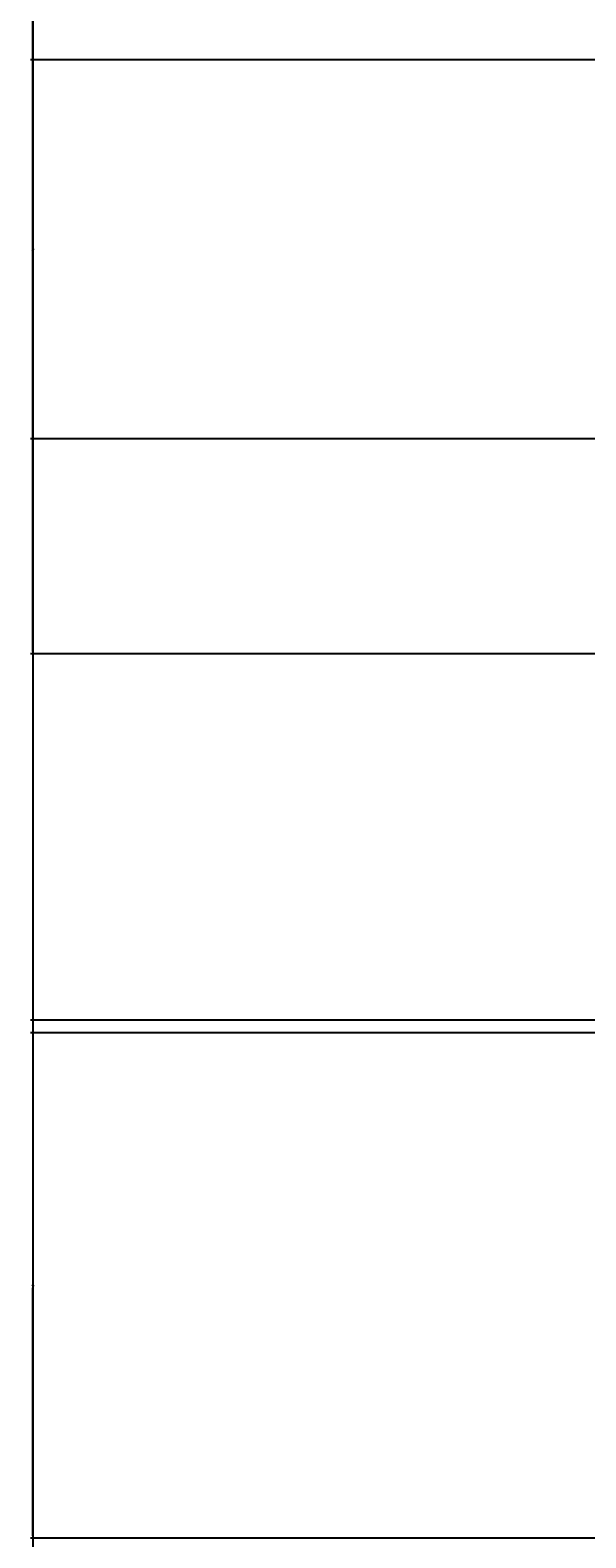
# Model space of a CAD drawing. Units: feet. Extents: x 105 to 1094, y -88 to 588.
# Tile 21 of 59: x 105 to 149, y 354 to 473. Entities that reach past the tile are written whole.
import ezdxf

# ---------------------------------------------------------------- set-up
doc = ezdxf.new("R2010")
doc.units = ezdxf.units.FT
doc.header["$MEASUREMENT"] = 0
doc.layers.add('A-ANNO-DIMS', color=2, linetype='Continuous', lineweight=18)
doc.styles.get("Standard").update_dxf_attribs({"font": 'arial.ttf'})
doc.dimstyles.get("Standard").update_dxf_attribs({"dimtxt": 0.18, "dimasz": 0.18, "dimexe": 0.18, "dimexo": 0.0625, "dimgap": 0.09, "dimtad": 0, "dimtih": 1, "dimtoh": 1, "dimdec": 4, "dimzin": 0, "dimdsep": 46, "dimtxsty": 'Standard', "dimcen": 0.09, "dimadec": 0, "dimazin": 0, "dimtfac": 1, "dimtdec": 4, "dimtofl": 0, "dimtmove": 0, "dimatfit": 3, "dimfxl": 1, "dimtolj": 1, "dimtzin": 0, "dimarcsym": 0})

# ---------------------------------------------------------------- blocks, each defined once
blk = doc.blocks.new('*D21')
at = {"layer": 'A-ANNO-DIMS', "color": 0, "lineweight": -2, "transparency": 16777216}
for p, q in [((849.63, 543.08), (105.46, 543.08)), ((105.64, 542.9), (105.64, 250.26)), ((105.64, -42.74), (105.64, 249.9)), ((849.63, -42.92), (105.46, -42.92))]:
    blk.add_line(p, q, dxfattribs=at)
at = {"layer": 'A-ANNO-DIMS', "color": 0, "transparency": 16777216}
for points in [[(105.61, 542.9), (105.67, 542.9), (105.64, 543.08)], [(105.61, -42.74), (105.67, -42.74), (105.64, -42.92)]]:
    blk.add_solid(points, dxfattribs=at)
at = {"layer": 'Defpoints', "color": 0, "transparency": 16777216}
for p in [(105.64, 543.08), (849.69, 543.08), (849.69, -42.92)]:
    blk.add_point(p, dxfattribs=at)
at = {"layer": 'A-ANNO-DIMS', "color": 0, "transparency": 16777216, "insert": (105.64, 250.08), "char_height": 0.18, "attachment_point": 5}
blk.add_mtext('\\A1;586', dxfattribs=at)
blk = doc.blocks.new('*D27')
at = {"layer": 'A-ANNO-DIMS', "color": 0, "lineweight": -2, "transparency": 16777216}
for p, q in [((231.63, 543.08), (105.46, 543.08)), ((105.64, 542.9), (105.64, 483.76)), ((105.64, 424.26), (105.64, 483.4)), ((150.63, 424.08), (105.46, 424.08))]:
    blk.add_line(p, q, dxfattribs=at)
at = {"layer": 'A-ANNO-DIMS', "color": 0, "transparency": 16777216}
for points in [[(105.61, 542.9), (105.67, 542.9), (105.64, 543.08)], [(105.61, 424.26), (105.67, 424.26), (105.64, 424.08)]]:
    blk.add_solid(points, dxfattribs=at)
at = {"layer": 'Defpoints', "color": 0, "transparency": 16777216}
for p in [(105.64, 543.08), (231.69, 543.08), (150.69, 424.08)]:
    blk.add_point(p, dxfattribs=at)
at = {"layer": 'A-ANNO-DIMS', "color": 0, "transparency": 16777216, "insert": (105.64, 483.58), "char_height": 0.18, "attachment_point": 5}
blk.add_mtext('\\A1;119', dxfattribs=at)
blk = doc.blocks.new('*D28')
at = {"layer": 'A-ANNO-DIMS', "color": 0, "lineweight": -2, "transparency": 16777216}
for p, q in [((150.63, 424.08), (105.46, 424.08)), ((105.64, 423.9), (105.64, 350.26)), ((105.64, 276.26), (105.64, 349.9)), ((150.63, 276.08), (105.46, 276.08))]:
    blk.add_line(p, q, dxfattribs=at)
at = {"layer": 'A-ANNO-DIMS', "color": 0, "transparency": 16777216}
for points in [[(105.61, 423.9), (105.67, 423.9), (105.64, 424.08)], [(105.61, 276.26), (105.67, 276.26), (105.64, 276.08)]]:
    blk.add_solid(points, dxfattribs=at)
at = {"layer": 'Defpoints', "color": 0, "transparency": 16777216}
for p in [(105.64, 424.08), (150.69, 424.08), (150.69, 276.08)]:
    blk.add_point(p, dxfattribs=at)
at = {"layer": 'A-ANNO-DIMS', "color": 0, "transparency": 16777216, "insert": (105.64, 350.08), "char_height": 0.18, "attachment_point": 5}
blk.add_mtext('\\A1;148', dxfattribs=at)
blk = doc.blocks.new('*D32')
at = {"layer": 'A-ANNO-DIMS', "color": 0, "lineweight": -2, "transparency": 16777216}
for p, q in [((646.63, 471.08), (105.46, 471.08)), ((105.64, 470.9), (105.64, 456.26)), ((105.64, 441.26), (105.64, 455.9)), ((646.63, 441.08), (105.46, 441.08))]:
    blk.add_line(p, q, dxfattribs=at)
at = {"layer": 'A-ANNO-DIMS', "color": 0, "transparency": 16777216}
for points in [[(105.61, 470.9), (105.67, 470.9), (105.64, 471.08)], [(105.61, 441.26), (105.67, 441.26), (105.64, 441.08)]]:
    blk.add_solid(points, dxfattribs=at)
at = {"layer": 'Defpoints', "color": 0, "transparency": 16777216}
for p in [(105.64, 471.08), (646.69, 471.08), (646.69, 441.08)]:
    blk.add_point(p, dxfattribs=at)
at = {"layer": 'A-ANNO-DIMS', "color": 0, "transparency": 16777216, "insert": (105.64, 456.08), "char_height": 0.18, "attachment_point": 5}
blk.add_mtext('\\A1;30', dxfattribs=at)
blk = doc.blocks.new('*D33')
at = {"layer": 'A-ANNO-DIMS', "color": 0, "lineweight": -2, "transparency": 16777216}
for p, q in [((646.63, 395.08), (105.46, 395.08)), ((105.64, 394.9), (105.64, 345.26)), ((105.64, 295.26), (105.64, 344.9)), ((646.63, 295.08), (105.46, 295.08))]:
    blk.add_line(p, q, dxfattribs=at)
at = {"layer": 'A-ANNO-DIMS', "color": 0, "transparency": 16777216}
for points in [[(105.61, 394.9), (105.67, 394.9), (105.64, 395.08)], [(105.61, 295.26), (105.67, 295.26), (105.64, 295.08)]]:
    blk.add_solid(points, dxfattribs=at)
at = {"layer": 'Defpoints', "color": 0, "transparency": 16777216}
for p in [(646.69, 395.08), (105.64, 295.08), (646.69, 295.08)]:
    blk.add_point(p, dxfattribs=at)
at = {"layer": 'A-ANNO-DIMS', "color": 0, "transparency": 16777216, "insert": (105.64, 345.08), "char_height": 0.18, "attachment_point": 5}
blk.add_mtext('\\A1;100', dxfattribs=at)
blk = doc.blocks.new('*D51')
at = {"layer": 'A-ANNO-DIMS', "color": 0, "lineweight": -2, "transparency": 16777216}
for p, q in [((432.63, 394.08), (105.46, 394.08)), ((105.64, 393.9), (105.64, 374.26)), ((105.64, 354.26), (105.64, 373.9)), ((426.63, 354.08), (105.46, 354.08))]:
    blk.add_line(p, q, dxfattribs=at)
at = {"layer": 'A-ANNO-DIMS', "color": 0, "transparency": 16777216}
for points in [[(105.61, 393.9), (105.67, 393.9), (105.64, 394.08)], [(105.61, 354.26), (105.67, 354.26), (105.64, 354.08)]]:
    blk.add_solid(points, dxfattribs=at)
at = {"layer": 'Defpoints', "color": 0, "transparency": 16777216}
for p in [(432.69, 394.08), (105.64, 354.08), (426.69, 354.08)]:
    blk.add_point(p, dxfattribs=at)
at = {"layer": 'A-ANNO-DIMS', "color": 0, "transparency": 16777216, "insert": (105.64, 374.08), "char_height": 0.18, "attachment_point": 5}
blk.add_mtext('\\A1;40', dxfattribs=at)

msp = doc.modelspace()

# ---------------------------------------------------------------- dimensions: what is measured, and where the dimension line sits
at = {"layer": 'A-ANNO-DIMS'}
for base, p1, p2, picture, middle in [((105.6383, 543.0812), (849.6883, -42.9188), (849.6883, 543.0812), '*D21', (105.6383, 250.0812)), ((105.6383, 543.0812), (150.6883, 424.0812), (231.6883, 543.0812), '*D27', (105.6383, 483.5812)), ((105.6383, 471.0812), (646.6883, 441.0812), (646.6883, 471.0812), '*D32', (105.6383, 456.0812)), ((105.6383, 424.0812), (150.6883, 276.0812), (150.6883, 424.0812), '*D28', (105.6383, 350.0812)), ((105.6383, 295.0812), (646.6883, 395.0812), (646.6883, 295.0812), '*D33', (105.6383, 345.0812)), ((105.6383, 354.0812), (432.6883, 394.0812), (426.6883, 354.0812), '*D51', (105.6383, 374.0812))]:
    dim = msp.add_linear_dim(base=base, p1=p1, p2=p2, angle=90, dimstyle='Standard', override={"dimdec": 0, "dimlfac": 1, "dimrnd": 0, "dimzin": 0, "dimdsep": 46, "dimlunit": 2}, dxfattribs=at)
    dim.commit()
    dim.dimension.update_dxf_attribs({"geometry": picture, "text_midpoint": middle})

doc.saveas('drawing.dxf')
